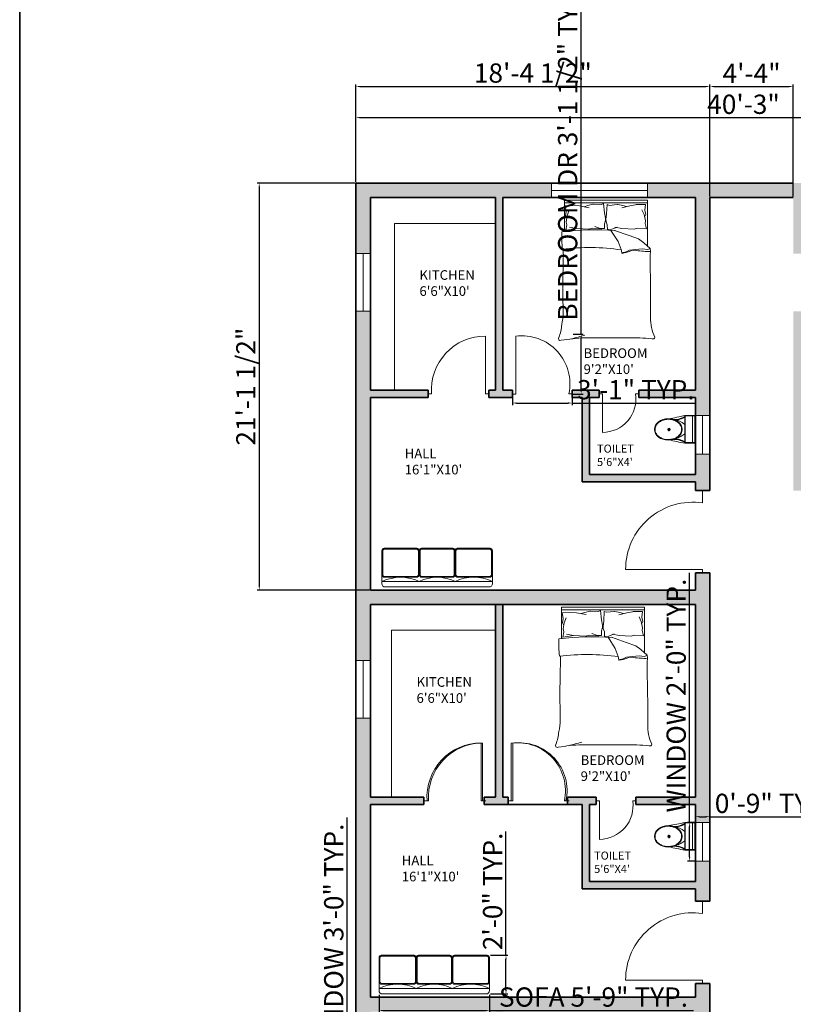
# Model space of a CAD drawing. Units: inches. Extents: x 1266 to 2869, y -408 to 3241.
# Tile 4 of 11: x 1266 to 1748, y 1767 to 2380. Entities that reach past the tile are written whole.
import ezdxf

# ---------------------------------------------------------------- set-up
doc = ezdxf.new("R2010")
doc.units = ezdxf.units.IN
for name, color, linetype, lineweight in [('A-ANNO-DIMS', 2, 'Continuous', 18), ('A-ANNO-TTLB', 7, 'Continuous', 35), ('A-AREA-IDEN', 7, 'Continuous', 18), ('A-DOOR', 4, 'Continuous', 18), ('A-FLOR-CASE', 9, 'Continuous', 18), ('A-FLOR-FIXT', 9, 'Continuous', 18), ('A-FURN', 8, 'Continuous', 18), ('A-GLAZ', 4, 'Continuous', 18), ('A-WALL', 7, 'Continuous', 35), ('A-WALL-PATT', 251, 'Continuous', 13)]:
    doc.layers.add(name, color=color, linetype=linetype, lineweight=lineweight)
doc.styles.get("Standard").update_dxf_attribs({"font": 'arial.ttf'})
doc.dimstyles.new('ISO-25', dxfattribs={"dimtxt": 12, "dimasz": 2.5, "dimexe": 1.25, "dimexo": 0.625, "dimtad": 1, "dimdec": 0, "dimlunit": 3, "dimtxsty": 'Standard', "dimcen": 2.5, "dimadec": 0, "dimazin": 0, "dimtfac": 1, "dimtdec": 0, "dimtmove": 0, "dimatfit": 3, "dimfxl": 1, "dimarcsym": 0})

# ---------------------------------------------------------------- blocks, each defined once
blk = doc.blocks.new('A$C31115884')
for p, q in [((283, 498), (223, 498)), ((258, 466), (258, 523)), ((0, 200), (0, 0)), ((520, 200), (0, 200)), ((10, 190), (10, 10)), ((510, 190), (10, 190)), ((510, 10), (510, 190)), ((520, 0), (520, 200)), ((510, 54), (0, 54)), ((10, 10), (510, 10)), ((0, 0), (520, 0))]:
    blk.add_line(p, q)
blk.add_circle((256, 496), 23.6)
for centre, radius, start, end in [((2778, -205), 2807, 165.4549, 171.7133), ((-295, 403), 365, 324.2091, 9.3499), ((-295, 403), 375, 324.2091, 9.3499), ((139, 406), 293, 315.8436, 2.6563), ((806, 403), 375, 179.2036, 215.7909), ((806, 403), 365, 170.6501, 215.7909), ((3237, 905), 2807, 188.2867, 194.5451), ((384, 406), 293, 190.2774, 224.1564)]:
    blk.add_arc(centre, radius, start, end)
blk.add_ellipse((256, 510), major_axis=(0, -261), ratio=0.772727)
blk.add_open_spline([(256, 259), (263, 259), (270, 260), (288, 262), (299, 265), (320, 273), (330, 278), (350, 291), (360, 299), (378, 316), (386, 326), (402, 347), (409, 358), (421, 383), (427, 395), (436, 422), (440, 436), (445, 465), (447, 480), (448, 509), (448, 524), (445, 553), (443, 568), (436, 596), (432, 610), (422, 636), (416, 649), (402, 672), (395, 683), (379, 703), (370, 712), (351, 728), (341, 735), (321, 746), (310, 751), (289, 757), (278, 759), (256, 761), (245, 761), (223, 757), (212, 754), (191, 746), (181, 741), (161, 728), (151, 720), (133, 703), (125, 693), (110, 672), (103, 660), (90, 636), (85, 623), (76, 596), (72, 582), (67, 553), (66, 538), (64, 509), (65, 494), (68, 465), (70, 450), (77, 422), (81, 408), (91, 382), (97, 370), (111, 346), (118, 335), (135, 316), (144, 307), (162, 291), (172, 284), (193, 273), (203, 269), (225, 262), (236, 260), (250, 259), (253, 259), (256, 259)], degree=3, knots=[0, 0, 0, 0, 0.110105, 0.110105, 0.285049, 0.285049, 0.459994, 0.459994, 0.634938, 0.634938, 0.809882, 0.809882, 0.984827, 0.984827, 1.159771, 1.159771, 1.334715, 1.334715, 1.50966, 1.50966, 1.684604, 1.684604, 1.859549, 1.859549, 2.034493, 2.034493, 2.209437, 2.209437, 2.384382, 2.384382, 2.559326, 2.559326, 2.73427, 2.73427, 2.909215, 2.909215, 3.084159, 3.084159, 3.259103, 3.259103, 3.434048, 3.434048, 3.608992, 3.608992, 3.783936, 3.783936, 3.958881, 3.958881, 4.133825, 4.133825, 4.30877, 4.30877, 4.483714, 4.483714, 4.658658, 4.658658, 4.833603, 4.833603, 5.008547, 5.008547, 5.183491, 5.183491, 5.358436, 5.358436, 5.53338, 5.53338, 5.708324, 5.708324, 5.883269, 5.883269, 6.058213, 6.058213, 6.233158, 6.233158, 6.283185, 6.283185, 6.283185, 6.283185])
blk = doc.blocks.new('*D2')
at = {"layer": 'A-ANNO-DIMS', "color": 0, "lineweight": -2, "transparency": 16777216}
for p, q in [((1475.69, 2278.97), (1475.69, 2320.42)), ((1478.19, 2319.17), (1956.19, 2319.17)), ((1958.69, 2278.97), (1958.69, 2320.42))]:
    blk.add_line(p, q, dxfattribs=at)
at = {"layer": 'A-ANNO-DIMS', "color": 0, "transparency": 16777216}
for points in [[(1478.19, 2319.59), (1478.19, 2318.76), (1475.69, 2319.17)], [(1956.19, 2319.59), (1956.19, 2318.76), (1958.69, 2319.17)]]:
    blk.add_solid(points, dxfattribs=at)
at = {"layer": 'Defpoints', "color": 0, "transparency": 16777216}
for p in [(1958.69, 2319.17), (1475.69, 2278.35), (1958.69, 2278.35)]:
    blk.add_point(p, dxfattribs=at)
at = {"layer": 'A-ANNO-DIMS', "color": 0, "transparency": 16777216, "insert": (1717.19, 2325.93), "char_height": 12, "attachment_point": 5}
blk.add_mtext('40\'-3"', dxfattribs=at)
blk = doc.blocks.new('BED-DOUBLE')
for p, q in [((3.76, 67.77), (3.76, 87.35)), ((3.76, 87.35), (55.42, 87.35)), ((55.42, 87.35), (55.42, 58.59)), ((3.76, 85.69), (55.42, 85.69)), ((4.21, 83.74), (8.84, 84.1)), ((4.21, 83.77), (4.84, 80.33)), ((4.84, 80.33), (4.37, 77.51)), ((5.46, 77.67), (6.55, 80.64)), ((8.84, 84.1), (8.96, 84.08)), ((8.96, 84.08), (13.09, 83.77)), ((13.09, 83.77), (19.03, 82.67)), ((16.06, 83.3), (18.25, 84.08)), ((18.25, 84.08), (21.37, 84.86)), ((21.37, 84.86), (21.72, 84.86)), ((21.72, 84.86), (26.53, 84.7)), ((26.53, 84.7), (28.09, 85.33)), ((28.09, 85.33), (28.71, 79.55)), ((30.24, 84.66), (29.98, 78.85)), ((31.84, 84.13), (30.24, 84.66)), ((36.63, 84.59), (31.84, 84.13)), ((36.98, 84.61), (36.63, 84.59)), ((40.14, 84.02), (36.98, 84.61)), ((45.31, 84.03), (39.45, 82.57)), ((42.38, 83.38), (40.14, 84.02)), ((49.42, 84.6), (45.31, 84.03)), ((54.17, 84.59), (48.33, 84.69)), ((48.33, 84.69), (49.42, 84.6)), ((53.3, 78.43), (52.03, 81.32)), ((54.17, 84.59), (53.76, 81.12)), ((53.76, 81.12), (54.41, 78.34)), ((4.37, 77.51), (4.99, 76.42)), ((4.84, 73.76), (5.46, 77.67)), ((5.15, 72.04), (4.84, 73.76)), ((28.71, 79.55), (29.34, 76.11)), ((29.34, 74.7), (28.71, 72.67)), ((29.34, 76.11), (29.34, 74.7)), ((29.98, 78.85), (29.57, 75.38)), ((29.57, 75.38), (29.66, 73.97)), ((29.66, 73.97), (30.41, 71.98)), ((54.17, 74.56), (53.3, 78.43)), ((54.41, 78.34), (53.85, 77.21)), ((53.97, 72.83), (54.17, 74.56)), ((4.52, 68.61), (5.15, 72.04)), ((10.03, 69.39), (4.52, 68.61)), ((6.9, 70.46), (11.26, 69.74)), ((11.26, 69.74), (10.03, 69.39)), ((11.26, 69.74), (18.84, 69.27)), ((18.84, 69.27), (20.95, 69.87)), ((20.95, 69.87), (26.5, 69.44)), ((26.06, 69.77), (22.66, 70.95)), ((28.71, 69.77), (26.06, 69.77)), ((28.71, 72.67), (28.71, 69.77)), ((30.41, 71.98), (30.59, 69.09)), ((30.59, 69.09), (33.24, 69.26)), ((32.71, 68.56), (37.24, 61.54)), ((33.24, 69.26), (36.56, 70.64)), ((43.94, 65.39), (34.92, 68.56)), ((35.2, 70.46), (39.56, 69.74)), ((39.56, 69.74), (47.14, 69.27)), ((47.14, 69.27), (49.26, 69.87)), ((49.26, 69.87), (54.81, 69.44)), ((54.81, 69.44), (53.97, 72.83)), ((37.24, 61.54), (39.08, 56.69)), ((49.96, 63.21), (43.94, 65.39)), ((53.15, 60.87), (49.96, 63.21)), ((39.08, 56.69), (39.42, 54.51)), ((42.1, 55.18), (44.27, 56.19)), ((44.27, 56.19), (47.96, 56.69)), ((47.96, 56.69), (52.14, 57.02)), ((52.14, 57.02), (55.49, 56.69)), ((57.15, 57.36), (53.15, 60.87)), ((55.49, 56.69), (57.15, 57.36)), ((57.24, 55.47), (57.15, 57.36, 4.18)), ((39.42, 54.51), (42.1, 55.18)), ((16.28, 1.69), (42.89, 1.69))]:
    blk.add_line(p, q)
for centre, radius, start, end in [((92.06, 65.63), 90.06, 178.72178, 185.60397), ((23.09, -109.45), 178.34, 86.08655, 96.78213), ((19.19, -81.63), 139.47, 81.78449, 96.90062), ((-180.86, 53.65), 183.89, 358.4762, 1.00819), ((33.68, 85.75), 32.06, 280.66171, 289.88058), ((47.29, 49.44), 6.73, 78.6608, 113.73842), ((55.49, 94.55), 39.11, 259.87628, 272.56571), ((197.03, 48.09), 139.99, 176.97912, 183.83645), ((39.6, 54.45), 0.199, 160.24637, 271.13765), ((524.11, 32.64), 521.39, 178.22771, 181.71854), ((-4874.07, 14.03), 4931.49, 0.00217, 0.28689), ((-29.08, 17.61), 32.04, 346.06484, 358.91125), ((82.33, 13.12), 24.93, 177.47136, 206.46809), ((-23.41, 11.38), 25.47, 337.97508, 356.652), ((1.18, 1.17), 1.18, 146.17358, 293.47814), ((23.16, -129.76), 131.62, 92.99578, 99.40907), ((-18.62, 112.98), 115.08, 283.38322, 287.70533), ((44.49, -142.13), 143.82, 84.4998, 90.63509), ((58.82, 2.09), 1.19, 242.65876, 356.02002)]:
    blk.add_arc(centre, radius, start, end)
blk = doc.blocks.new('SOFA-3-SEAT')
for points in [[(0, 22.36), (0, 7.74, 0.414214), (1.72, 6.02), (21.5, 6.02, 0.414214), (23.22, 7.74), (23.22, 22.36, 0.414214), (21.5, 24.08), (1.72, 24.08, 0.414214)], [(0.52, 22.36), (0.52, 7.74, 0.414214), (1.72, 6.54), (21.5, 6.54, 0.414214), (22.7, 7.74), (22.7, 22.36, 0.414214), (21.5, 23.56), (1.72, 23.56, 0.414214)], [(45.57, 22.36), (45.57, 7.74, -0.414214), (43.85, 6.02), (24.94, 6.02, -0.414214), (23.22, 7.74), (23.22, 22.36, -0.414214), (24.94, 24.08), (43.85, 24.08, -0.414214)], [(45.06, 22.36), (45.06, 7.74, -0.414214), (43.85, 6.54), (24.94, 6.54, -0.414214), (23.73, 7.74), (23.73, 22.36, -0.414214), (24.94, 23.56), (43.85, 23.56, -0.414214)], [(45.57, 22.36), (45.57, 7.74, 0.414214), (47.29, 6.02), (67.07, 6.02, 0.414214), (68.79, 7.74), (68.79, 22.36, 0.414214), (67.07, 24.08), (47.29, 24.08, 0.414214)], [(46.09, 22.36), (46.09, 7.74, 0.414214), (47.29, 6.54), (67.07, 6.54, 0.414214), (68.27, 7.74), (68.27, 22.36, 0.414214), (67.07, 23.56), (47.29, 23.56, 0.414214)]]:
    blk.add_lwpolyline(points, format="xyb", close=True)
at = {"ltscale": 0.03}
blk.add_lwpolyline([(21.82, 24.08), (1.38, 24.08, 0.414214), (0, 22.7), (0, 2.06, 0.414214), (2.06, 0), (66.73, 0, 0.414214), (68.79, 2.06), (68.79, 22.7, 0.414214), (67.41, 24.08), (46.97, 24.08, 0.414214), (45.59, 22.7, -1), (45.56, 22.7, 0.414214), (44.18, 24.08), (24.61, 24.08, 0.414214), (23.23, 22.7, -1), (23.2, 22.7, 0.414214)], format="xyb", close=True, dxfattribs=at)
blk.add_lwpolyline([(0, 3.44), (68.79, 3.44)])
for centre, radius, start, end in [((11.61, -21.35), 27.38, 64.91063, 115.08937), ((34.4, -19.35), 25.38, 63.869, 116.131), ((57.18, -21.07), 27.12, 64.65382, 115.34618)]:
    blk.add_arc(centre, radius, start, end)
blk = doc.blocks.new('DOOR-KITCHEN-L')
for p, q in [((35.61, 0), (35.61, 36)), ((0, 0), (2, 0)), ((37.61, 0), (35.61, 0))]:
    blk.add_line(p, q)
blk.add_arc((35.61, 2.31), 33.69, 90, 183.92625)
blk = doc.blocks.new('DOOR-BEDROOM-L')
for p, q in [((2, 0), (2, 36)), ((0, 0), (2, 0)), ((37.12, 0.11), (35.12, 0.11))]:
    blk.add_line(p, q)
blk.add_arc((5.98, 6.45), 29.82, 347.72217, 97.67592)
blk = doc.blocks.new('DOOR-BATH-L')
for p, q in [((0, 24), (2, 24)), ((2, 24), (2, 0)), ((24.7, 24), (22.7, 24))]:
    blk.add_line(p, q)
blk.add_arc((2, 20.92), 20.92, 270, 8.45113)
blk = doc.blocks.new('DOOR-ENTRY-L')
for p, q in [((48, 51.27), (48, 45.59)), ((48, 45.59), (48, 43.59)), ((12, 2), (0, 2)), ((48, 2), (12, 2)), ((48, 0), (48, 2))]:
    blk.add_line(p, q)
blk.add_arc((42.02, 2), 42.02, 81.81164, 180)
blk = doc.blocks.new('WIN-PLAN-60')
for p, q in [((0, 9), (0, 0)), ((60, 4.5), (60, 9)), ((60, 9), (60, 0)), ((0, 4.5), (60, 4.5)), ((0, 0), (0, 4.5))]:
    blk.add_line(p, q)
blk = doc.blocks.new('WIN-PLAN-36')
for p, q in [((0, 36), (9, 36)), ((4.5, 36), (4.5, 0)), ((9, 36), (4.5, 36)), ((4.5, 0), (0, 0)), ((0, 0), (9, 0))]:
    blk.add_line(p, q)
blk = doc.blocks.new('WIN-PLAN-36-2')
for p, q in [((0, 36), (9, 36)), ((4.5, 36), (4.5, 0)), ((9, 36), (4.5, 36)), ((2.69, 0), (0, 0)), ((0, 0), (9, 0))]:
    blk.add_line(p, q)
blk = doc.blocks.new('WIN-PLAN-24-2')
for p, q in [((0, 24), (9, 24)), ((4.5, 24), (4.5, 0)), ((9, 24), (4.5, 24)), ((4.5, 0), (0, 0)), ((0, 0), (9, 0))]:
    blk.add_line(p, q)
blk = doc.blocks.new('WIN-PLAN-24-3')
for p, q in [((0, 24), (9, 24)), ((4.5, 24), (4.5, 0)), ((9, 24), (4.5, 24)), ((2.69, 0), (0, 0)), ((0, 0), (9, 0))]:
    blk.add_line(p, q)
blk = doc.blocks.new('COUNTER-KITCHEN-2')
for p, q in [((0, 0), (0, 103.95)), ((0, 103.95), (63, 103.95))]:
    blk.add_line(p, q)
blk = doc.blocks.new('COUNTER-KITCHEN-3')
for p, q in [((0, 0), (0, 103.95)), ((0, 103.95), (64.81, 103.95))]:
    blk.add_line(p, q)
blk = doc.blocks.new('*D31')
at = {"layer": 'A-ANNO-DIMS', "color": 0, "lineweight": -2, "transparency": 16777216}
for p, q in [((1470.29, 1727.52), (1470.29, 1883.12)), ((1475.07, 1727.52), (1469.04, 1727.52)), ((1470.29, 1694.02), (1470.29, 1725.02)), ((1475.07, 1691.52), (1469.04, 1691.52))]:
    blk.add_line(p, q, dxfattribs=at)
at = {"layer": 'A-ANNO-DIMS', "color": 0, "transparency": 16777216}
for points in [[(1469.88, 1725.02), (1470.71, 1725.02), (1470.29, 1727.52)], [(1469.88, 1694.02), (1470.71, 1694.02), (1470.29, 1691.52)]]:
    blk.add_solid(points, dxfattribs=at)
at = {"layer": 'Defpoints', "color": 0, "transparency": 16777216}
for p in [(1470.29, 1727.52), (1475.69, 1727.52), (1475.69, 1691.52)]:
    blk.add_point(p, dxfattribs=at)
at = {"layer": 'A-ANNO-DIMS', "color": 0, "transparency": 16777216, "insert": (1463.45, 1806.57), "char_height": 12, "attachment_point": 5, "rotation": 90}
blk.add_mtext('WINDOW 3\'-0" TYP.', dxfattribs=at)
blk = doc.blocks.new('*D53')
at = {"layer": 'A-ANNO-DIMS', "color": 0, "lineweight": -2, "transparency": 16777216}
for p, q in [((1616.02, 2184.29), (1616.02, 2408.76)), ((1611.05, 2184.29), (1617.27, 2184.29)), ((1616.02, 2149.49), (1616.02, 2181.79)), ((1611.05, 2146.99), (1617.27, 2146.99))]:
    blk.add_line(p, q, dxfattribs=at)
at = {"layer": 'A-ANNO-DIMS', "color": 0, "transparency": 16777216}
for points in [[(1615.6, 2181.79), (1616.43, 2181.79), (1616.02, 2184.29)], [(1615.6, 2149.49), (1616.43, 2149.49), (1616.02, 2146.99)]]:
    blk.add_solid(points, dxfattribs=at)
at = {"layer": 'Defpoints', "color": 0, "transparency": 16777216}
for p in [(1610.42, 2184.29), (1616.02, 2184.29), (1610.42, 2146.99)]:
    blk.add_point(p, dxfattribs=at)
at = {"layer": 'A-ANNO-DIMS', "color": 0, "transparency": 16777216, "insert": (1609.18, 2297.78), "char_height": 12, "attachment_point": 5, "rotation": 90}
blk.add_mtext('BEDROOM DR 3\'-1 1/2" TYP.', dxfattribs=at)
blk = doc.blocks.new('*D54')
at = {"layer": 'A-ANNO-DIMS', "color": 0, "lineweight": -2, "transparency": 16777216}
for p, q in [((1573.23, 2146.37), (1573.23, 2140.15)), ((1575.73, 2141.4), (1607.92, 2141.4)), ((1610.42, 2146.37), (1610.42, 2140.15)), ((1610.42, 2141.4), (1687.31, 2141.4))]:
    blk.add_line(p, q, dxfattribs=at)
at = {"layer": 'A-ANNO-DIMS', "color": 0, "transparency": 16777216}
for points in [[(1575.73, 2141.81), (1575.73, 2140.98), (1573.23, 2141.4)], [(1607.92, 2141.81), (1607.92, 2140.98), (1610.42, 2141.4)]]:
    blk.add_solid(points, dxfattribs=at)
at = {"layer": 'Defpoints', "color": 0, "transparency": 16777216}
for p in [(1573.23, 2146.99), (1610.42, 2146.99), (1610.42, 2141.4)]:
    blk.add_point(p, dxfattribs=at)
at = {"layer": 'A-ANNO-DIMS', "color": 0, "transparency": 16777216, "insert": (1650.11, 2148.15), "char_height": 12, "attachment_point": 5}
blk.add_mtext('3\'-1" TYP.', dxfattribs=at)
blk = doc.blocks.new('*D67')
at = {"layer": 'A-ANNO-DIMS', "color": 0, "lineweight": -2, "transparency": 16777216}
for p, q in [((1490.09, 1772.67), (1490.09, 1761.73)), ((1558.88, 1772.67), (1558.88, 1761.73)), ((1492.59, 1762.98), (1556.38, 1762.98)), ((1558.88, 1762.98), (1686.02, 1762.98))]:
    blk.add_line(p, q, dxfattribs=at)
at = {"layer": 'A-ANNO-DIMS', "color": 0, "transparency": 16777216}
for points in [[(1492.59, 1763.4), (1492.59, 1762.56), (1490.09, 1762.98)], [(1556.38, 1763.4), (1556.38, 1762.56), (1558.88, 1762.98)]]:
    blk.add_solid(points, dxfattribs=at)
at = {"layer": 'Defpoints', "color": 0, "transparency": 16777216}
for p in [(1490.09, 1773.3), (1558.88, 1773.3), (1558.88, 1762.98)]:
    blk.add_point(p, dxfattribs=at)
at = {"layer": 'A-ANNO-DIMS', "color": 0, "transparency": 16777216, "insert": (1623.7, 1769.81), "char_height": 12, "attachment_point": 5}
blk.add_mtext('SOFA 5\'-9" TYP.', dxfattribs=at)
blk = doc.blocks.new('*D68')
at = {"layer": 'A-ANNO-DIMS', "color": 0, "lineweight": -2, "transparency": 16777216}
for p, q in [((1569.19, 1797.38), (1569.19, 1874.48)), ((1559.5, 1797.38), (1570.44, 1797.38)), ((1569.19, 1775.8), (1569.19, 1794.88)), ((1559.5, 1773.3), (1570.44, 1773.3))]:
    blk.add_line(p, q, dxfattribs=at)
at = {"layer": 'A-ANNO-DIMS', "color": 0, "transparency": 16777216}
for points in [[(1568.78, 1794.88), (1569.61, 1794.88), (1569.19, 1797.38)], [(1568.78, 1775.8), (1569.61, 1775.8), (1569.19, 1773.3)]]:
    blk.add_solid(points, dxfattribs=at)
at = {"layer": 'Defpoints', "color": 0, "transparency": 16777216}
for p in [(1558.88, 1797.38), (1569.19, 1797.38), (1558.88, 1773.3)]:
    blk.add_point(p, dxfattribs=at)
at = {"layer": 'A-ANNO-DIMS', "color": 0, "transparency": 16777216, "insert": (1562.44, 1837.18), "char_height": 12, "attachment_point": 5, "rotation": 90}
blk.add_mtext('2\'-0" TYP.', dxfattribs=at)
blk = doc.blocks.new('*D77')
at = {"layer": 'A-ANNO-DIMS', "color": 0, "lineweight": -2, "transparency": 16777216}
for p, q in [((1683.59, 1880.11), (1683.59, 2035.71)), ((1686.57, 1880.11), (1682.34, 1880.11)), ((1683.59, 1858.61), (1683.59, 1877.61)), ((1686.57, 1856.11), (1682.34, 1856.11))]:
    blk.add_line(p, q, dxfattribs=at)
at = {"layer": 'A-ANNO-DIMS', "color": 0, "transparency": 16777216}
for points in [[(1683.18, 1877.61), (1684.01, 1877.61), (1683.59, 1880.11)], [(1683.18, 1858.61), (1684.01, 1858.61), (1683.59, 1856.11)]]:
    blk.add_solid(points, dxfattribs=at)
at = {"layer": 'Defpoints', "color": 0, "transparency": 16777216}
for p in [(1683.59, 1880.11), (1687.19, 1880.11), (1687.19, 1856.11)]:
    blk.add_point(p, dxfattribs=at)
at = {"layer": 'A-ANNO-DIMS', "color": 0, "transparency": 16777216, "insert": (1676.76, 1959.16), "char_height": 12, "attachment_point": 5, "rotation": 90}
blk.add_mtext('WINDOW 2\'-0" TYP.', dxfattribs=at)
blk = doc.blocks.new('*D78')
at = {"layer": 'A-ANNO-DIMS', "color": 0, "lineweight": -2, "transparency": 16777216}
for p, q in [((1687.19, 1880.73), (1687.19, 1884.96)), ((1689.69, 1883.71), (1693.69, 1883.71)), ((1696.19, 1880.73), (1696.19, 1884.96)), ((1696.19, 1883.71), (1773.09, 1883.71))]:
    blk.add_line(p, q, dxfattribs=at)
at = {"layer": 'A-ANNO-DIMS', "color": 0, "transparency": 16777216}
for points in [[(1689.69, 1884.13), (1689.69, 1883.29), (1687.19, 1883.71)], [(1693.69, 1884.13), (1693.69, 1883.29), (1696.19, 1883.71)]]:
    blk.add_solid(points, dxfattribs=at)
at = {"layer": 'Defpoints', "color": 0, "transparency": 16777216}
for p in [(1696.19, 1883.71), (1687.19, 1880.11), (1696.19, 1880.11)]:
    blk.add_point(p, dxfattribs=at)
at = {"layer": 'A-ANNO-DIMS', "color": 0, "transparency": 16777216, "insert": (1735.89, 1890.46), "char_height": 12, "attachment_point": 5}
blk.add_mtext('0\'-9" TYP.', dxfattribs=at)
blk = doc.blocks.new('*D81')
at = {"layer": 'A-ANNO-DIMS', "color": 0, "lineweight": -2, "transparency": 16777216}
for p, q in [((1475.69, 2278.97), (1475.69, 2339.8)), ((1478.19, 2338.55), (1693.69, 2338.55)), ((1696.19, 2269.97), (1696.19, 2339.8))]:
    blk.add_line(p, q, dxfattribs=at)
at = {"layer": 'A-ANNO-DIMS', "color": 0, "transparency": 16777216}
for points in [[(1478.19, 2338.96), (1478.19, 2338.13), (1475.69, 2338.55)], [(1693.69, 2338.96), (1693.69, 2338.13), (1696.19, 2338.55)]]:
    blk.add_solid(points, dxfattribs=at)
at = {"layer": 'Defpoints', "color": 0, "transparency": 16777216}
for p in [(1696.19, 2338.55), (1475.69, 2278.35), (1696.19, 2269.35)]:
    blk.add_point(p, dxfattribs=at)
at = {"layer": 'A-ANNO-DIMS', "color": 0, "transparency": 16777216, "insert": (1585.94, 2345.38), "char_height": 12, "attachment_point": 5}
blk.add_mtext('18\'-4 1/2"', dxfattribs=at)
blk = doc.blocks.new('*D82')
at = {"layer": 'A-ANNO-DIMS', "color": 0, "lineweight": -2, "transparency": 16777216}
for p, q in [((1696.19, 2269.97), (1696.19, 2339.8)), ((1698.69, 2338.55), (1745.69, 2338.55)), ((1748.19, 2269.97), (1748.19, 2339.8))]:
    blk.add_line(p, q, dxfattribs=at)
at = {"layer": 'A-ANNO-DIMS', "color": 0, "transparency": 16777216}
for points in [[(1698.69, 2338.96), (1698.69, 2338.13), (1696.19, 2338.55)], [(1745.69, 2338.96), (1745.69, 2338.13), (1748.19, 2338.55)]]:
    blk.add_solid(points, dxfattribs=at)
at = {"layer": 'Defpoints', "color": 0, "transparency": 16777216}
for p in [(1748.19, 2338.55), (1696.19, 2269.35), (1748.19, 2269.35)]:
    blk.add_point(p, dxfattribs=at)
at = {"layer": 'A-ANNO-DIMS', "color": 0, "transparency": 16777216, "insert": (1722.19, 2345.17), "char_height": 12, "attachment_point": 5}
blk.add_mtext('4\'-4"', dxfattribs=at)
blk = doc.blocks.new('*D83')
at = {"layer": 'A-ANNO-DIMS', "color": 0, "lineweight": -2, "transparency": 16777216}
for p, q in [((1475.07, 2278.35), (1414.24, 2278.35)), ((1415.49, 2275.85), (1415.49, 2027.35)), ((1484.07, 2024.85), (1414.24, 2024.85))]:
    blk.add_line(p, q, dxfattribs=at)
at = {"layer": 'A-ANNO-DIMS', "color": 0, "transparency": 16777216}
for points in [[(1415.08, 2275.85), (1415.91, 2275.85), (1415.49, 2278.35)], [(1415.08, 2027.35), (1415.91, 2027.35), (1415.49, 2024.85)]]:
    blk.add_solid(points, dxfattribs=at)
at = {"layer": 'Defpoints', "color": 0, "transparency": 16777216}
for p in [(1475.69, 2278.35), (1415.49, 2024.85), (1484.69, 2024.85)]:
    blk.add_point(p, dxfattribs=at)
at = {"layer": 'A-ANNO-DIMS', "color": 0, "transparency": 16777216, "insert": (1408.66, 2151.6), "char_height": 12, "attachment_point": 5, "rotation": 90}
blk.add_mtext('21\'-1 1/2"', dxfattribs=at)

msp = doc.modelspace()

# ---------------------------------------------------------------- hatches: boundary and pattern name
at = {"layer": 'A-WALL-PATT'}
h = msp.add_hatch(color=256, dxfattribs=at)
h.dxf.hatch_style = 1
h.paths.add_polyline_path([(1484.69, 2269.35), (1562.69, 2269.35), (1562.69, 2149.35), (1558.42, 2149.35), (1558.42, 2144.85), (1567.19, 2144.85), (1573.23, 2144.85), (1573.23, 2146.74), (1573.23, 2149.35), (1567.19, 2149.35), (1567.19, 2269.35), (1597.45, 2269.35), (1597.45, 2273.85), (1597.45, 2278.35), (1475.69, 2278.35), (1475.69, 2234.52), (1484.69, 2234.52)])
h.paths.add_polyline_path([(1873.25, 2278.35), (1748.19, 2278.35), (1696.19, 2278.35), (1657.45, 2278.35), (1657.45, 2269.35), (1687.19, 2269.35), (1687.19, 2149.35), (1651.94, 2149.35), (1651.94, 2144.85), (1687.19, 2144.85), (1687.19, 2133.61), (1696.19, 2133.61), (1696.19, 2269.35), (1748.19, 2269.35), (1748.19, 2234.52), (1757.19, 2234.52), (1757.19, 2269.35), (1835.19, 2269.35), (1835.19, 2149.35), (1827.33, 2149.35), (1827.33, 2144.85), (1843.74, 2144.85), (1843.74, 2149.35), (1839.69, 2149.35), (1839.69, 2269.35), (1873.25, 2269.35), (1873.25, 2273.85)])
h.paths.add_polyline_path([(1958.69, 2278.35), (1933.25, 2278.35), (1933.25, 2269.35), (1949.69, 2269.35), (1949.69, 2149.35), (1912.22, 2149.35), (1912.22, 2144.85), (1949.69, 2144.85), (1949.69, 2133.61), (1958.69, 2133.61)])
h.paths.add_polyline_path([(1883.69, 2144.85), (1889.08, 2144.85), (1889.08, 2149.35), (1875.58, 2149.35), (1875.58, 2144.85), (1879.19, 2144.85), (1879.19, 2092.35), (1949.69, 2092.35), (1949.69, 2086.89), (1949.69, 2024.85), (1933.25, 2024.85), (1933.25, 2015.85), (1949.69, 2015.85), (1949.69, 1895.85), (1912.45, 1895.85), (1912.45, 1891.35), (1949.69, 1891.35), (1949.69, 1880.11), (1958.69, 1880.11), (1958.69, 2086.89), (1958.69, 2109.61), (1949.69, 2109.61), (1949.69, 2096.85), (1883.69, 2096.85)])
h.paths.add_polyline_path([(1757.19, 2198.52), (1748.19, 2198.52), (1748.19, 2086.89), (1757.19, 2086.89), (1757.19, 2144.85), (1793.55, 2144.85), (1793.55, 2149.35), (1757.19, 2149.35)])
h.paths.add_polyline_path([(1696.19, 2109.61), (1687.19, 2109.61), (1687.19, 2096.85), (1621.19, 2096.85), (1621.19, 2144.85), (1627.24, 2144.85), (1627.24, 2149.35), (1616.69, 2149.35), (1610.35, 2149.35), (1610.35, 2144.85), (1616.69, 2144.85), (1616.69, 2092.35), (1687.19, 2092.35), (1687.19, 2086.89), (1696.19, 2086.89)], flags=17)
h.paths.add_polyline_path([(1484.69, 2144.85), (1520.8, 2144.85), (1520.8, 2149.35), (1484.69, 2149.35), (1484.69, 2198.52), (1475.69, 2198.52), (1475.69, 1981.02), (1484.69, 1981.02), (1484.69, 2015.85), (1687.19, 2015.85), (1687.19, 1895.85), (1650.13, 1895.85), (1650.13, 1891.35), (1687.19, 1891.35), (1687.19, 1880.11), (1696.19, 1880.11), (1696.19, 2035.62), (1687.19, 2035.62), (1687.19, 2024.85), (1484.69, 2024.85)])
h.paths.add_polyline_path([(1484.69, 1691.52), (1475.69, 1691.52), (1475.69, 1474.02), (1484.69, 1474.02)])
h.paths.add_polyline_path([(1518.03, 1895.85), (1484.69, 1895.85), (1484.69, 1945.02), (1475.69, 1945.02), (1475.69, 1727.52), (1484.69, 1727.52), (1484.69, 1762.35), (1687.19, 1762.35), (1687.19, 1642.35), (1651.94, 1642.35), (1651.94, 1637.85), (1687.19, 1637.85), (1687.19, 1589.85), (1621.19, 1589.85), (1621.19, 1637.85), (1627.19, 1637.85), (1627.19, 1642.35), (1610.89, 1642.35), (1610.89, 1637.85), (1616.69, 1637.85), (1616.69, 1585.35), (1687.19, 1585.35), (1687.19, 1579.45), (1696.19, 1579.45), (1696.19, 1779.84), (1687.19, 1779.84), (1687.19, 1771.35), (1484.69, 1771.35), (1484.69, 1891.35), (1518.03, 1891.35)])
h.paths.add_polyline_path([(1567.19, 2015.85), (1562.69, 2015.85), (1562.69, 1895.85), (1555.64, 1895.85), (1555.64, 1891.35), (1570.46, 1891.35), (1570.46, 1895.85), (1567.19, 1895.85)], flags=17)
h.paths.add_polyline_path([(1625.43, 1895.85), (1607.58, 1895.85), (1607.58, 1891.35), (1616.69, 1891.35), (1616.69, 1838.85), (1687.19, 1838.85), (1687.19, 1831.11), (1696.19, 1831.11), (1696.19, 1856.11), (1687.19, 1856.11), (1687.19, 1843.35), (1621.19, 1843.35), (1621.19, 1891.35), (1625.43, 1891.35)], flags=17)
h.paths.add_polyline_path([(1567.19, 1762.35), (1562.69, 1762.35), (1562.69, 1642.35), (1558.42, 1642.35), (1558.42, 1637.85), (1573.23, 1637.85), (1573.23, 1642.35), (1567.19, 1642.35)], flags=17)
h.paths.add_polyline_path([(1520.8, 1642.35), (1484.69, 1642.35), (1484.69, 1637.85), (1520.8, 1637.85)], flags=17)
h.paths.add_polyline_path([(1687.19, 1517.85), (1484.69, 1517.85), (1484.69, 1508.85), (1562.69, 1508.85), (1562.69, 1388.85), (1567.19, 1388.85), (1567.19, 1508.85), (1687.19, 1508.85)])
h.paths.add_polyline_path([(1696.19, 1528.18), (1687.19, 1528.18), (1687.19, 1323.21), (1696.19, 1323.21)])
h.paths.add_polyline_path([(1696.19, 1271.94), (1687.19, 1271.94), (1687.19, 1264.35), (1484.69, 1264.35), (1484.69, 1283.77), (1480.19, 1283.77), (1475.69, 1283.77), (1475.69, 1255.35), (1480.19, 1255.35), (1696.19, 1255.35)])
h.paths.add_polyline_path([(1484.69, 1438.02), (1475.69, 1438.02), (1475.69, 1319.77), (1484.69, 1319.77)])
h.paths.add_polyline_path([(1873.25, 1513.35), (1873.25, 1517.85), (1757.19, 1517.85), (1757.19, 1528.62), (1748.19, 1528.62), (1748.19, 1474.02), (1757.19, 1474.02), (1757.19, 1508.85), (1835.19, 1508.85), (1835.19, 1388.85), (1827.33, 1388.85), (1827.33, 1384.35), (1843.74, 1384.35), (1843.74, 1388.85), (1839.69, 1388.85), (1839.69, 1508.85), (1873.25, 1508.85)])
h.paths.add_polyline_path([(1958.69, 1602.61), (1949.69, 1602.61), (1949.69, 1517.85), (1933.25, 1517.85), (1933.25, 1508.85), (1949.69, 1508.85), (1949.69, 1388.85), (1912.22, 1388.85), (1912.22, 1384.35), (1949.69, 1384.35), (1949.69, 1373.11), (1958.69, 1373.11)])
h.paths.add_polyline_path([(1958.69, 1349.11), (1949.69, 1349.11), (1949.69, 1336.35), (1883.69, 1336.35), (1883.69, 1384.35), (1889.08, 1384.35), (1889.08, 1388.85), (1875.58, 1388.85), (1875.58, 1384.35), (1879.19, 1384.35), (1879.19, 1331.85), (1949.69, 1331.85), (1949.69, 1315.59), (1958.69, 1315.59)])
h.paths.add_polyline_path([(1958.69, 1279.59), (1954.19, 1279.59), (1949.69, 1279.59), (1949.69, 1264.35), (1757.19, 1264.35), (1757.19, 1275.12), (1748.19, 1275.12), (1748.19, 1255.35), (1958.69, 1255.35)])
h.paths.add_polyline_path([(1757.19, 1438.02), (1748.19, 1438.02), (1748.19, 1326.39), (1757.19, 1326.39)])
h.paths.add_polyline_path([(1793.55, 1388.85), (1757.19, 1388.85), (1757.19, 1384.35), (1793.55, 1384.35)], flags=0)

# ---------------------------------------------------------------- linework, layer by layer
at = {"layer": 'A-ANNO-TTLB'}
msp.add_lwpolyline([(1266.23, 3241.34), (2868.62, 3241.34), (2868.62, 986.84), (1266.23, 986.84)], close=True, dxfattribs=at)
at = {"layer": 'A-FURN'}
for points in [[(1491.9, 2049.16), (1491.9, 2034.54, 0.414214), (1493.62, 2032.82), (1513.4, 2032.82, 0.414214), (1515.12, 2034.54), (1515.12, 2049.16, 0.414214), (1513.4, 2050.88), (1493.62, 2050.88, 0.414214)], [(1492.42, 2049.16), (1492.42, 2034.54, 0.414214), (1493.62, 2033.33), (1513.4, 2033.33, 0.414214), (1514.6, 2034.54), (1514.6, 2049.16, 0.414214), (1513.4, 2050.36), (1493.62, 2050.36, 0.414214)], [(1537.47, 2049.16), (1537.47, 2034.54, -0.414214), (1535.75, 2032.82), (1516.84, 2032.82, -0.414214), (1515.12, 2034.54), (1515.12, 2049.16, -0.414214), (1516.84, 2050.88), (1535.75, 2050.88, -0.414214)], [(1536.96, 2049.16), (1536.96, 2034.54, -0.414214), (1535.75, 2033.33), (1516.84, 2033.33, -0.414214), (1515.63, 2034.54), (1515.63, 2049.16, -0.414214), (1516.84, 2050.36), (1535.75, 2050.36, -0.414214)], [(1537.47, 2049.16), (1537.47, 2034.54, 0.414214), (1539.19, 2032.82), (1558.97, 2032.82, 0.414214), (1560.69, 2034.54), (1560.69, 2049.16, 0.414214), (1558.97, 2050.88), (1539.19, 2050.88, 0.414214)], [(1537.99, 2049.16), (1537.99, 2034.54, 0.414214), (1539.19, 2033.33), (1558.97, 2033.33, 0.414214), (1560.18, 2034.54), (1560.18, 2049.16, 0.414214), (1558.97, 2050.36), (1539.19, 2050.36, 0.414214)]]:
    msp.add_lwpolyline(points, format="xyb", close=True, dxfattribs=at)
at = {"layer": 'A-FURN', "ltscale": 0.03}
msp.add_lwpolyline([(1513.72, 2050.88), (1493.28, 2050.88, 0.414214), (1491.9, 2049.5), (1491.9, 2028.86, 0.414214), (1493.96, 2026.8), (1558.63, 2026.8, 0.414214), (1560.69, 2028.86), (1560.69, 2049.5, 0.414214), (1559.32, 2050.88), (1538.87, 2050.88, 0.414214), (1537.49, 2049.5, -1), (1537.46, 2049.5, 0.414214), (1536.08, 2050.88), (1516.51, 2050.88, 0.414214), (1515.13, 2049.5, -1), (1515.1, 2049.5, 0.414214)], format="xyb", close=True, dxfattribs=at)
at = {"layer": 'A-FURN'}
msp.add_lwpolyline([(1491.9, 2030.24), (1560.69, 2030.24)], dxfattribs=at)
for centre, radius, start, end in [((1503.51, 2005.45), 27.38, 64.91063, 115.08937), ((1526.3, 2007.45), 25.38, 63.869, 116.131), ((1549.08, 2005.73), 27.12, 64.65382, 115.34618)]:
    msp.add_arc(centre, radius, start, end, dxfattribs=at)
at = {"layer": 'A-WALL'}
for p, q in [((1475.69, 2278.35), (1475.69, 1255.35)), ((1475.69, 2278.35), (1696.19, 2278.35)), ((1696.19, 2278.35), (1748.19, 2278.35)), ((1484.69, 2269.35), (1562.69, 2269.35)), ((1484.69, 2269.35), (1484.69, 2149.35)), ((1562.69, 2269.35), (1562.69, 2149.35)), ((1567.19, 2269.35), (1567.19, 2149.35)), ((1567.19, 2269.35), (1687.19, 2269.35)), ((1687.19, 2269.35), (1687.19, 2149.35)), ((1696.19, 2269.35), (1696.19, 2086.89)), ((1748.19, 2269.35), (1696.19, 2269.35)), ((1484.69, 2149.35), (1520.8, 2149.35)), ((1520.8, 2149.35), (1520.8, 2144.85)), ((1558.42, 2149.35), (1558.42, 2144.85)), ((1558.42, 2149.35), (1562.69, 2149.35)), ((1567.19, 2149.35), (1573.23, 2149.35)), ((1573.23, 2149.35), (1573.23, 2146.74)), ((1573.23, 2146.74), (1573.23, 2144.85)), ((1616.69, 2149.35), (1610.35, 2149.35)), ((1610.35, 2149.35), (1610.35, 2144.85)), ((1616.69, 2149.35), (1627.24, 2149.35)), ((1627.24, 2149.35), (1627.24, 2144.85)), ((1651.94, 2149.35), (1651.94, 2144.85)), ((1651.94, 2149.35), (1687.19, 2149.35)), ((1484.69, 2144.85), (1520.8, 2144.85)), ((1484.69, 2144.85), (1484.69, 2024.85)), ((1558.42, 2144.85), (1567.19, 2144.85)), ((1573.23, 2144.85), (1567.19, 2144.85)), ((1610.35, 2144.85), (1616.69, 2144.85)), ((1616.69, 2144.85), (1616.69, 2092.35)), ((1621.19, 2144.85), (1621.19, 2096.85)), ((1621.19, 2144.85), (1627.24, 2144.85)), ((1651.94, 2144.85), (1687.19, 2144.85)), ((1687.19, 2144.85), (1687.19, 2096.85)), ((1616.69, 2092.35), (1687.19, 2092.35)), ((1621.19, 2096.85), (1687.19, 2096.85)), ((1687.19, 2092.35), (1687.19, 2086.89)), ((1687.19, 2086.89), (1696.19, 2086.89)), ((1687.19, 2035.62), (1696.19, 2035.62)), ((1687.19, 2035.62), (1687.19, 2024.85)), ((1696.19, 2035.62), (1696.19, 1831.11)), ((1484.69, 2024.85), (1687.19, 2024.85)), ((1484.69, 2015.85), (1687.19, 2015.85)), ((1484.69, 2015.85), (1484.69, 1895.85)), ((1562.69, 2015.85), (1562.69, 1895.85)), ((1567.19, 2015.85), (1567.19, 1895.85)), ((1687.19, 2015.85), (1687.19, 1895.85)), ((1484.69, 1895.85), (1518.03, 1895.85)), ((1518.03, 1893.6), (1518.03, 1895.85)), ((1518.03, 1895.85), (1518.03, 1891.35)), ((1555.64, 1895.85), (1555.64, 1891.35)), ((1555.64, 1895.85), (1562.69, 1895.85)), ((1567.19, 1895.85), (1570.46, 1895.85)), ((1570.46, 1893.49), (1570.46, 1895.85)), ((1570.46, 1895.85), (1570.46, 1891.35)), ((1607.58, 1893.6), (1607.58, 1895.85)), ((1607.58, 1895.85), (1607.58, 1891.35)), ((1625.43, 1895.85), (1607.58, 1895.85)), ((1625.43, 1891.35), (1625.43, 1895.85)), ((1625.43, 1895.85), (1625.43, 1895.85)), ((1650.13, 1893.6), (1650.13, 1895.85)), ((1650.13, 1895.85), (1650.13, 1891.35)), ((1650.13, 1895.85), (1687.19, 1895.85)), ((1484.69, 1891.35), (1518.03, 1891.35)), ((1484.69, 1891.35), (1484.69, 1771.35)), ((1555.64, 1891.35), (1616.69, 1891.35)), ((1616.69, 1891.35), (1616.69, 1838.85)), ((1621.19, 1891.35), (1621.19, 1843.35)), ((1621.19, 1891.35), (1625.43, 1891.35)), ((1650.13, 1891.35), (1687.19, 1891.35)), ((1687.19, 1891.35), (1687.19, 1843.35)), ((1621.19, 1843.35), (1687.19, 1843.35)), ((1616.69, 1838.85), (1687.19, 1838.85)), ((1687.19, 1838.85), (1687.19, 1831.11)), ((1691.69, 1831.11), (1687.19, 1831.11)), ((1687.19, 1831.11), (1696.19, 1831.11)), ((1687.19, 1779.84), (1687.19, 1779.84)), ((1687.19, 1779.84), (1696.19, 1779.84)), ((1687.19, 1779.84), (1687.19, 1771.35)), ((1696.19, 1779.84), (1696.19, 1579.45)), ((1484.69, 1771.35), (1687.19, 1771.35))]:
    msp.add_line(p, q, dxfattribs=at)

# ---------------------------------------------------------------- block references
at = {"layer": 'A-DOOR'}
for name, p in [('DOOR-BEDROOM-L', (1573.23, 2146.99)), ('DOOR-KITCHEN-L', (1520.8, 2147.1)), ('DOOR-BATH-L', (1627.24, 2123.1)), ('DOOR-ENTRY-L', (1643.69, 2035.62)), ('DOOR-KITCHEN-L', (1518.03, 1893.6)), ('DOOR-KITCHEN-L', (1518.99, 1893.6)), ('DOOR-BEDROOM-L', (1570.46, 1893.49)), ('DOOR-BEDROOM-L', (1571.42, 1893.49)), ('DOOR-BATH-L', (1625.43, 1869.6)), ('DOOR-BATH-L', (1625.43, 1869.6)), ('DOOR-ENTRY-L', (1643.69, 1779.84))]:
    msp.add_blockref(name, p, dxfattribs=at)
at = {"layer": 'A-FLOR-CASE'}
for name, p in [('COUNTER-KITCHEN-2', (1499.69, 2149.35)), ('COUNTER-KITCHEN-3', (1497.88, 1895.85))]:
    msp.add_blockref(name, p, dxfattribs=at)
at = {"layer": 'A-FLOR-FIXT', "xscale": 0.0330640103915726, "yscale": 0.0330640103915726, "zscale": 0.0330640103915726, "rotation": 89.99999999999996}
for p in [(1687.19, 2116.46), (1687.19, 1862.96)]:
    msp.add_blockref('A$C31115884', p, dxfattribs=at)
at = {"layer": 'A-FURN'}
for name, p in [('BED-DOUBLE', (1601.89, 2180.39)), ('BED-DOUBLE', (1600.07, 1926.89)), ('SOFA-3-SEAT', (1490.09, 1773.3))]:
    msp.add_blockref(name, p, dxfattribs=at)
at = {"layer": 'A-GLAZ'}
for name, p in [('WIN-PLAN-60', (1597.45, 2269.35)), ('WIN-PLAN-36', (1475.69, 2198.52)), ('WIN-PLAN-24-2', (1687.19, 2109.61)), ('WIN-PLAN-36-2', (1475.69, 1945.02)), ('WIN-PLAN-24-3', (1687.19, 1856.11))]:
    msp.add_blockref(name, p, dxfattribs=at)

# ---------------------------------------------------------------- texts
at = {"layer": 'A-AREA-IDEN', "attachment_point": 1}
for s, width, insert, char_height in [('KITCHEN\\P6\'6"X10\'', 112.1355, (1515.28, 2224.14), 6), ('BEDROOM\\P9\'2"X10\'', 62.026, (1617.54, 2175.46), 6), ('HALL\\P16\'1"X10\'', 100.9767, (1506.1, 2112.93), 6), ('TOILET\\P5\'6"X4\'', 46.3569, (1625.93, 2115.49), 5), ('KITCHEN\\P6\'6"X10\'', 112.1355, (1513.47, 1970.64), 6), ('BEDROOM\\P9\'2"X10\'', 62.026, (1615.72, 1921.96), 6), ('HALL\\P16\'1"X10\'', 100.9767, (1504.28, 1859.43), 6), ('TOILET\\P5\'6"X4\'', 46.3569, (1624.12, 1861.99), 5)]:
    msp.add_mtext_dynamic_manual_height_columns(s, width=width, gutter_width=12.5, heights=[0], dxfattribs=dict(at, insert=insert, char_height=char_height))

# ---------------------------------------------------------------- dimensions: what is measured, and where the dimension line sits
at = {"layer": 'A-ANNO-DIMS'}
for base, p1, p2, text, picture, middle in [((1616.02, 2184.29), (1610.42, 2146.99), (1610.42, 2184.29), 'BEDROOM DR <> TYP.', '*D53', (1609.18, 2297.78)), ((1683.59, 1880.11), (1687.19, 1856.11), (1687.19, 1880.11), 'WINDOW <> TYP.', '*D77', (1676.76, 1959.16)), ((1470.29, 1727.52), (1475.69, 1691.52), (1475.69, 1727.52), 'WINDOW <> TYP.', '*D31', (1463.45, 1806.57)), ((1569.19, 1797.38), (1558.88, 1773.3), (1558.88, 1797.38), '<> TYP.', '*D68', (1562.44, 1837.18))]:
    dim = msp.add_linear_dim(base=base, p1=p1, p2=p2, angle=90, text=text, dimstyle='ISO-25', override={"dimdec": 1, "dimlfac": 1, "dimrnd": 0, "dimzin": 1, "dimdsep": 46, "dimlunit": 4, "dimfrac": 2}, dxfattribs=at)
    dim.commit()
    dim.dimension.update_dxf_attribs({"geometry": picture, "text_midpoint": middle})
for base, p1, p2, picture, middle in [((1696.19, 2338.55), (1475.69, 2278.35), (1696.19, 2269.35), '*D81', (1585.94, 2345.38)), ((1748.19, 2338.55), (1696.19, 2269.35), (1748.19, 2269.35), '*D82', (1722.19, 2345.17))]:
    dim = msp.add_linear_dim(base=base, p1=p1, p2=p2, dimstyle='ISO-25', override={"dimdec": 1, "dimlfac": 1, "dimrnd": 0, "dimzin": 1, "dimdsep": 46, "dimlunit": 4, "dimfrac": 2}, dxfattribs=at)
    dim.commit()
    dim.dimension.update_dxf_attribs({"geometry": picture, "text_midpoint": middle})
dim = msp.add_linear_dim(base=(1958.69, 2319.17), p1=(1475.69, 2278.35), p2=(1958.69, 2278.35), dimstyle='ISO-25', override={"dimclrd": 0, "dimclre": 0, "dimclrt": 0}, dxfattribs=at)
dim.commit()
dim.dimension.update_dxf_attribs({"geometry": '*D2', "text_midpoint": (1717.19, 2319.17), "dimtype": 160})
dim = msp.add_linear_dim(base=(1415.49, 2024.85), p1=(1475.69, 2278.35), p2=(1484.69, 2024.85), angle=90, dimstyle='ISO-25', override={"dimdec": 1, "dimlfac": 1, "dimrnd": 0, "dimzin": 1, "dimdsep": 46, "dimlunit": 4, "dimfrac": 2}, dxfattribs=at)
dim.commit()
dim.dimension.update_dxf_attribs({"geometry": '*D83', "text_midpoint": (1408.66, 2151.6)})
for base, p1, p2, text, picture, middle in [((1610.42, 2141.4), (1573.23, 2146.99), (1610.42, 2146.99), '<> TYP.', '*D54', (1650.11, 2148.15)), ((1696.19, 1883.71), (1687.19, 1880.11), (1696.19, 1880.11), '<> TYP.', '*D78', (1735.89, 1890.46)), ((1558.88, 1762.98), (1490.09, 1773.3), (1558.88, 1773.3), 'SOFA <> TYP.', '*D67', (1623.7, 1769.81))]:
    dim = msp.add_linear_dim(base=base, p1=p1, p2=p2, text=text, dimstyle='ISO-25', override={"dimdec": 1, "dimlfac": 1, "dimrnd": 0, "dimzin": 1, "dimdsep": 46, "dimlunit": 4, "dimfrac": 2}, dxfattribs=at)
    dim.commit()
    dim.dimension.update_dxf_attribs({"geometry": picture, "text_midpoint": middle})

doc.saveas('drawing.dxf')
